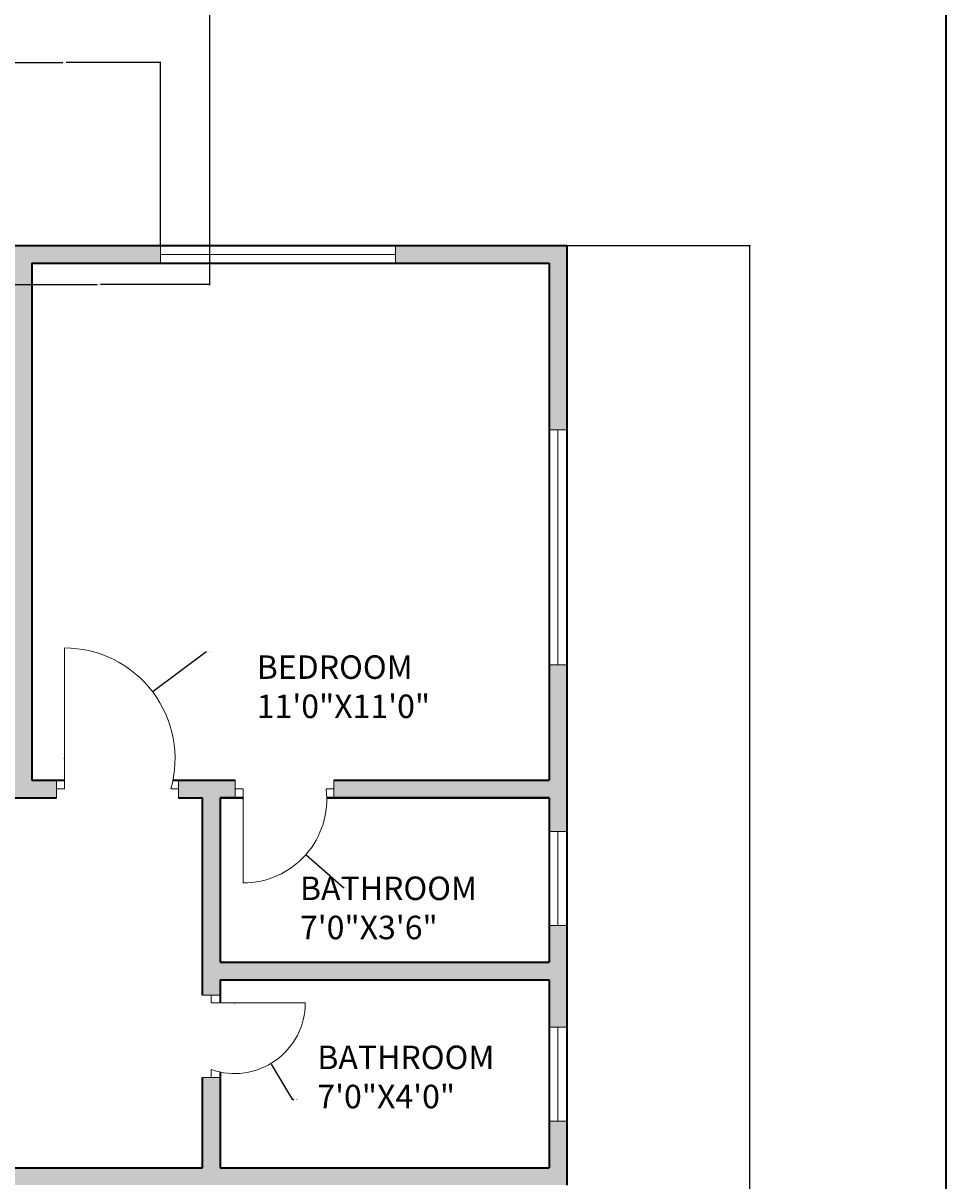
# Model space of a CAD drawing. Units: inches. Extents: x 2314 to 3223, y 1382 to 2735.
# Tile 13 of 14: x 2987 to 3223, y 2143 to 2439. Entities that reach past the tile are written whole.
import ezdxf

# ---------------------------------------------------------------- set-up
doc = ezdxf.new("R2010")
doc.units = ezdxf.units.IN
for name, color, linetype, lineweight in [('A-ANNO-DIMS', 2, 'Continuous', 18), ('A-ANNO-TTLB', 7, 'Continuous', 35), ('A-AREA-IDEN', 7, 'Continuous', 18), ('A-DOOR', 3, 'Continuous', 18), ('A-GLAZ', 4, 'Continuous', 18), ('A-WALL', 7, 'Continuous', 35)]:
    doc.layers.add(name, color=color, linetype=linetype, lineweight=lineweight)
doc.layers.add('A-WALL-PATT', color=251, linetype='Continuous', lineweight=13, true_color=0x636466)
doc.styles.get("Standard").update_dxf_attribs({"font": 'arial.ttf'})
doc.dimstyles.get("Standard").update_dxf_attribs({"dimtxt": 0.18, "dimasz": 0.18, "dimexe": 0.18, "dimexo": 0.0625, "dimgap": 0.09, "dimtad": 0, "dimtih": 1, "dimtoh": 1, "dimdec": 4, "dimzin": 0, "dimdsep": 46, "dimtxsty": 'Standard', "dimcen": 0.09, "dimadec": 0, "dimazin": 0, "dimtfac": 1, "dimtdec": 4, "dimtofl": 0, "dimtmove": 0, "dimatfit": 3, "dimfxl": 1, "dimtolj": 1, "dimtzin": 0, "dimarcsym": 0})

# ---------------------------------------------------------------- blocks, each defined once
blk = doc.blocks.new('WIN-PLAN-24')
for p, q in [((0, 24), (4.5, 24)), ((4.5, 24), (2.25, 24)), ((2.25, 24), (2.25, 0)), ((2.25, 0), (0, 0)), ((0, 0), (4.5, 0))]:
    blk.add_line(p, q)
blk = doc.blocks.new('WIN-PLAN-60')
for p, q in [((0, 4.5), (0, 0)), ((60, 2.25), (60, 4.5)), ((60, 4.5), (60, 0)), ((0, 0), (0, 2.25)), ((0, 2.25), (60, 2.25))]:
    blk.add_line(p, q)
blk = doc.blocks.new('*D30')
at = {"layer": 'A-ANNO-DIMS', "color": 0, "lineweight": -2, "transparency": 16777216}
for p, q in [((3125.96, 2381.78), (3172.77, 2381.78)), ((3172.59, 2381.6), (3172.59, 1973.38)), ((3172.59, 1564.8), (3172.59, 1973.02)), ((2822.96, 1564.62), (3172.77, 1564.62))]:
    blk.add_line(p, q, dxfattribs=at)
at = {"layer": 'A-ANNO-DIMS', "color": 0, "transparency": 16777216}
for points in [[(3172.56, 2381.6), (3172.62, 2381.6), (3172.59, 2381.78)], [(3172.56, 1564.8), (3172.62, 1564.8), (3172.59, 1564.62)]]:
    blk.add_solid(points, dxfattribs=at)
at = {"layer": 'Defpoints', "color": 0, "transparency": 16777216}
for p in [(3125.89, 2381.78), (2822.89, 1564.62), (3172.59, 1564.62)]:
    blk.add_point(p, dxfattribs=at)
at = {"layer": 'A-ANNO-DIMS', "color": 0, "transparency": 16777216, "insert": (3172.59, 1973.2), "char_height": 0.18, "attachment_point": 5}
blk.add_mtext('\\A1;817.2', dxfattribs=at)
blk = doc.blocks.new('*D45')
at = {"layer": 'A-ANNO-DIMS', "color": 0, "lineweight": -2, "transparency": 16777216}
for p, q in [((2973.21, 2381.85), (2973.21, 2428.66)), ((2973.39, 2428.48), (2997.29, 2428.48)), ((3021.98, 2428.48), (2998.08, 2428.48)), ((3022.16, 2381.85), (3022.16, 2428.66))]:
    blk.add_line(p, q, dxfattribs=at)
at = {"layer": 'A-ANNO-DIMS', "color": 0, "transparency": 16777216}
for points in [[(2973.39, 2428.51), (2973.39, 2428.45), (2973.21, 2428.48)], [(3021.98, 2428.51), (3021.98, 2428.45), (3022.16, 2428.48)]]:
    blk.add_solid(points, dxfattribs=at)
at = {"layer": 'Defpoints', "color": 0, "transparency": 16777216}
for p in [(3022.16, 2428.48), (2973.21, 2381.78), (3022.16, 2381.78)]:
    blk.add_point(p, dxfattribs=at)
at = {"layer": 'A-ANNO-DIMS', "color": 0, "transparency": 16777216, "insert": (2997.69, 2428.48), "char_height": 0.18, "attachment_point": 5}
blk.add_mtext('\\A1;48.95', dxfattribs=at)
blk = doc.blocks.new('*D59')
at = {"layer": 'A-ANNO-DIMS', "color": 0, "lineweight": -2, "transparency": 16777216}
for p, q in [((2978.22, 2502.62), (2978.22, 2371.63)), ((3034.7, 2502.62), (3034.7, 2371.63)), ((2978.4, 2371.81), (3006.07, 2371.81)), ((3034.52, 2371.81), (3006.85, 2371.81))]:
    blk.add_line(p, q, dxfattribs=at)
at = {"layer": 'A-ANNO-DIMS', "color": 0, "transparency": 16777216}
for points in [[(2978.4, 2371.84), (2978.4, 2371.78), (2978.22, 2371.81)], [(3034.52, 2371.84), (3034.52, 2371.78), (3034.7, 2371.81)]]:
    blk.add_solid(points, dxfattribs=at)
at = {"layer": 'Defpoints', "color": 0, "transparency": 16777216}
for p in [(2978.22, 2502.68), (3034.7, 2502.68), (3034.7, 2371.81)]:
    blk.add_point(p, dxfattribs=at)
at = {"layer": 'A-ANNO-DIMS', "color": 0, "transparency": 16777216, "insert": (3006.46, 2371.81), "char_height": 0.18, "attachment_point": 5}
blk.add_mtext('\\A1;56.47', dxfattribs=at)
blk = doc.blocks.new('*D74')
at = {"layer": 'A-ANNO-DIMS', "color": 0, "lineweight": -2, "transparency": 16777216}
for p, q in [((3033.74, 2278), (3020.36, 2267.91)), ((3033.92, 2278), (3033.74, 2278)), ((2997.58, 2250.79), (2997.76, 2250.79)), ((2997.67, 2250.7), (2997.67, 2250.88))]:
    blk.add_line(p, q, dxfattribs=at)
at = {"layer": 'A-ANNO-DIMS', "color": 0, "transparency": 16777216}
blk.add_solid([(3020.34, 2267.93), (3020.38, 2267.88), (3020.21, 2267.8)], dxfattribs=at)
at = {"layer": 'Defpoints', "color": 0, "transparency": 16777216}
for p in [(3020.21, 2267.8), (2997.67, 2250.79)]:
    blk.add_point(p, dxfattribs=at)
at = {"layer": 'A-ANNO-DIMS', "color": 0, "transparency": 16777216, "insert": (3034.4, 2278), "char_height": 0.18, "attachment_point": 5}
blk.add_mtext('\\A1;R28.24', dxfattribs=at)
blk = doc.blocks.new('*D86')
at = {"layer": 'A-ANNO-DIMS', "color": 0, "lineweight": -2, "transparency": 16777216}
for p, q in [((3043.27, 2240.32), (3043.27, 2240.5)), ((3043.18, 2240.41), (3043.36, 2240.41)), ((3068.89, 2217.76), (3059.42, 2226.13)), ((3069.07, 2217.76), (3068.89, 2217.76))]:
    blk.add_line(p, q, dxfattribs=at)
at = {"layer": 'A-ANNO-DIMS', "color": 0, "transparency": 16777216}
blk.add_solid([(3059.44, 2226.16), (3059.4, 2226.11), (3059.29, 2226.25)], dxfattribs=at)
at = {"layer": 'Defpoints', "color": 0, "transparency": 16777216}
for p in [(3043.27, 2240.41), (3059.29, 2226.25)]:
    blk.add_point(p, dxfattribs=at)
at = {"layer": 'A-ANNO-DIMS', "color": 0, "transparency": 16777216, "insert": (3069.62, 2217.76), "char_height": 0.18, "attachment_point": 5}
blk.add_mtext('\\A1;R21.375', dxfattribs=at)
blk = doc.blocks.new('*D91')
at = {"layer": 'A-ANNO-DIMS', "color": 0, "lineweight": -2, "transparency": 16777216}
for p, q in [((3041.01, 2188.4), (3041.19, 2188.4)), ((3041.1, 2188.31), (3041.1, 2188.49)), ((3056.02, 2163.69), (3050.52, 2172.8)), ((3056.2, 2163.69), (3056.02, 2163.69))]:
    blk.add_line(p, q, dxfattribs=at)
at = {"layer": 'A-ANNO-DIMS', "color": 0, "transparency": 16777216}
blk.add_solid([(3050.54, 2172.82), (3050.49, 2172.79), (3050.42, 2172.96)], dxfattribs=at)
at = {"layer": 'Defpoints', "color": 0, "transparency": 16777216}
for p in [(3041.1, 2188.4), (3050.42, 2172.96)]:
    blk.add_point(p, dxfattribs=at)
at = {"layer": 'A-ANNO-DIMS', "color": 0, "transparency": 16777216, "insert": (3056.75, 2163.69), "char_height": 0.18, "attachment_point": 5}
blk.add_mtext('\\A1;R18.042', dxfattribs=at)

msp = doc.modelspace()

# ---------------------------------------------------------------- hatches: boundary and pattern name
at = {"layer": 'A-WALL-PATT'}
h = msp.add_hatch(color=256, dxfattribs=at)
h.dxf.hatch_style = 1
h.paths.add_polyline_path([(2443.3302, 2379.5332), (2443.3302, 2381.7832), (2410.3927, 2381.7832), (2410.3927, 2336.7008), (2414.8927, 2336.7008), (2414.8927, 2377.2832), (2443.3302, 2377.2832)])
h.paths.add_polyline_path([(2561.3645, 2379.5332), (2561.3645, 2381.7832), (2503.3302, 2381.7832), (2503.3302, 2377.2832), (2546.8927, 2377.2832), (2546.8927, 2245.2832), (2541.8787, 2245.2832), (2541.8787, 2240.7832), (2551.3927, 2240.7832), (2551.3927, 2377.2832), (2561.3645, 2377.2832)])
h.paths.add_polyline_path([(2656.0607, 2381.7832), (2597.3645, 2381.7832), (2597.3645, 2377.2832), (2617.3927, 2377.2832), (2617.3927, 2257.2832), (2584.2532, 2257.2832), (2584.2532, 2252.7832), (2625.8528, 2252.7832), (2625.8528, 2255.0332), (2625.8528, 2257.2832), (2621.8927, 2257.2832), (2621.8927, 2377.2832), (2656.0607, 2377.2832), (2656.0607, 2379.5332)])
h.paths.add_polyline_path([(2807.3418, 2381.7832), (2716.0607, 2381.7832), (2716.0607, 2377.2832), (2765.8927, 2377.2832), (2765.8927, 2257.2832), (2661.6935, 2257.2832), (2661.6935, 2252.7832), (2765.8927, 2252.7832), (2765.8927, 2146.2832), (2760.9259, 2146.2832), (2760.9259, 2141.8832), (2775.7119, 2141.8832), (2775.7119, 2146.2832), (2770.3927, 2146.2832), (2770.3927, 2252.7832), (2877.684, 2252.7832), (2877.684, 2255.0332), (2877.684, 2257.2832), (2770.3927, 2257.2832), (2770.3927, 2377.2832), (2807.3418, 2377.2832), (2807.3418, 2379.5332)])
h.paths.add_polyline_path([(2937.2118, 2381.7832), (2867.3418, 2381.7832), (2867.3418, 2377.2832), (2914.3927, 2377.2832), (2914.3927, 2257.2832), (2908.4124, 2257.2832), (2908.4124, 2252.7832), (2960.6432, 2252.7832), (2960.6432, 2255.0332), (2960.6432, 2257.2832), (2918.8927, 2257.2832), (2918.8927, 2377.2832), (2937.2118, 2377.2832)])
h.paths.add_polyline_path([(3022.1601, 2381.7832), (2973.2118, 2381.7832), (2973.2118, 2379.5332), (2973.2118, 2377.2832), (2984.8927, 2377.2832), (2984.8927, 2257.2832), (2980.0601, 2257.2832), (2980.0601, 2252.7832), (2984.8927, 2252.7832), (2984.8927, 2240.7832), (2995.668, 2240.7832), (2995.668, 2243.0332), (2995.668, 2245.2832), (2989.3927, 2245.2832), (2989.3927, 2377.2832), (3022.1601, 2377.2832), (3022.1601, 2379.5332)])
h.paths.add_polyline_path([(3125.8927, 2381.7832), (3082.1601, 2381.7832), (3082.1601, 2377.2832), (3121.3927, 2377.2832), (3121.3927, 2334.7388), (3125.8927, 2334.7388)])
h.paths.add_polyline_path([(3125.8927, 2274.7388), (3121.3927, 2274.7388), (3121.3927, 2245.2832), (3066.4832, 2245.2832), (3066.4832, 2240.7832), (3121.3927, 2240.7832), (3121.3927, 2232.1868), (3125.8927, 2232.1868)])
h.paths.add_polyline_path([(3125.8927, 2208.1868), (3121.3927, 2208.1868), (3121.3927, 2198.7832), (3037.3927, 2198.7832), (3037.3927, 2240.7832), (3041.2694, 2240.7832), (3041.2694, 2243.0332), (3041.2694, 2245.2832), (3026.8205, 2245.2832), (3026.8205, 2240.7832), (3032.8927, 2240.7832), (3032.8927, 2190.4022), (3037.3927, 2190.4022), (3037.3927, 2194.2832), (3121.3927, 2194.2832), (3121.3927, 2182.1835), (3125.8927, 2182.1835)])
h.paths.add_polyline_path([(3125.8927, 2158.1835), (3121.3927, 2158.1835), (3121.3927, 2146.2832), (3037.3927, 2146.2832), (3037.3927, 2169.3726), (3035.1427, 2169.3726), (3032.8927, 2169.3726), (3032.8927, 2146.2832), (2812.7301, 2146.2832), (2812.7301, 2144.0832), (2812.7301, 2141.8832), (2818.3927, 2141.8832), (2818.3927, 1970.1316), (2822.8927, 1970.1316), (2822.8927, 1978.8832), (2903.9846, 1978.8832), (2903.9846, 1981.1332), (2903.9846, 1983.3832), (2822.8927, 1983.3832), (2822.8927, 2115.3832), (2851.7162, 2115.3832), (2851.7162, 2117.6332), (2851.7162, 2119.8832), (2822.8927, 2119.8832), (2822.8927, 2141.8832), (3125.8927, 2141.8832)])
h.paths.add_polyline_path([(3125.8927, 2119.8832), (3081.193, 2119.8832), (3081.193, 2115.3832), (3121.3927, 2115.3832), (3121.3927, 2071.8188), (3125.8927, 2071.8188)], flags=17)
h.paths.add_polyline_path([(2989.3927, 2115.3832), (3021.193, 2115.3832), (3021.193, 2117.6332), (3021.193, 2119.8832), (2979.123, 2119.8832), (2979.123, 2115.3832), (2984.8927, 2115.3832), (2984.8927, 2019.3832), (2981.9225, 2019.3832), (2981.9225, 2014.8832), (2984.8927, 2014.8832), (2984.8927, 1983.3832), (2984.8927, 1978.8832), (2989.3927, 1978.8832), (2989.3927, 1983.3832)], flags=17)
h.paths.add_polyline_path([(2947.3927, 2115.3832), (2955.123, 2115.3832), (2955.123, 2117.6332), (2955.123, 2119.8832), (2911.7162, 2119.8832), (2911.7162, 2115.3832), (2942.8927, 2115.3832), (2942.8927, 1983.3832), (2936.7017, 1983.3832), (2936.7017, 1978.8832), (2947.3927, 1978.8832), (2947.3927, 1983.3832), (2947.3927, 2014.8832), (2960.7167, 2014.8832), (2960.7167, 2017.1332), (2960.7167, 2019.3832), (2947.3927, 2019.3832)], flags=17)
h.paths.add_polyline_path([(3037.3927, 1978.8832), (3041.8276, 1978.8832), (3041.8276, 1981.1332), (3041.8276, 1983.3832), (3025.477, 1983.3832), (3025.477, 1978.8832), (3032.8927, 1978.8832), (3032.8927, 1927.1259), (3035.1427, 1927.1259), (3037.3927, 1927.1259)])
h.paths.add_polyline_path([(3125.8927, 2011.8188), (3123.6427, 2011.8188), (3121.3927, 2011.8188), (3121.3927, 1983.3832), (3065, 1983.3832), (3065, 1978.8832), (3121.3927, 1978.8832), (3121.3927, 1970.5932), (3125.8927, 1970.5932)], flags=17)
h.paths.add_polyline_path([(2994.2341, 1983.3832), (2989.3927, 1983.3832), (2989.3927, 1978.8832), (2994.2341, 1978.8832), (2994.2341, 1981.1332)], flags=16)
h.paths.add_polyline_path([(3125.8927, 1946.5932), (3121.3927, 1946.5932), (3121.3927, 1936.8832), (3037.3927, 1936.8832), (3037.3927, 1932.3832), (3121.3927, 1932.3832), (3121.3927, 1919.825), (3125.8927, 1919.825)])
h.paths.add_polyline_path([(3125.8927, 1883.825), (3121.3927, 1883.825), (3121.3927, 1866.3832), (3037.3927, 1866.3832), (3037.3927, 1899.0954), (3035.1427, 1899.0954), (3032.8927, 1899.0954), (3032.8927, 1866.3832), (2822.8927, 1866.3832), (2822.8927, 1938.7212), (2820.6427, 1938.7212), (2818.3927, 1938.7212), (2818.3927, 1786.9239), (2822.8927, 1786.9239), (2822.8927, 1861.8832), (3032.8927, 1861.8832), (3032.8927, 1825.1023), (3037.3927, 1825.1023), (3037.3927, 1861.8832), (3121.3927, 1861.8832), (3121.3927, 1844.6765), (3125.8927, 1844.6765)])
h.paths.add_polyline_path([(3125.8927, 1808.6765), (3121.3927, 1808.6765), (3121.3927, 1795.8832), (3037.3927, 1795.8832), (3037.3927, 1799.4755), (3032.8927, 1799.4755), (3032.8927, 1749.3832), (3026.5034, 1749.3832), (3026.5034, 1744.8832), (3032.8927, 1744.8832), (3034.9255, 1744.8832), (3043.1326, 1744.8832), (3043.1326, 1747.1332), (3043.1326, 1749.3832), (3037.3927, 1749.3832), (3037.3927, 1791.3832), (3121.3927, 1791.3832), (3121.3927, 1783.3103), (3125.8927, 1783.3103)])
h.paths.add_polyline_path([(3125.8927, 1759.3103), (3121.3927, 1759.3103), (3121.3927, 1749.3832), (3065.1845, 1749.3832), (3065.1845, 1744.8832), (3121.3927, 1744.8832), (3121.3927, 1709.3573), (3125.8927, 1709.3573)])
h.paths.add_polyline_path([(3125.8927, 1649.3573), (3121.3927, 1649.3573), (3121.3927, 1612.8832), (3095.116, 1612.8832), (3095.116, 1608.3832), (3125.8927, 1608.3832)])
h.paths.add_polyline_path([(3035.116, 1612.8832), (2993.8927, 1612.8832), (2993.8927, 1744.8832), (2998.7409, 1744.8832), (2998.7409, 1749.3832), (2989.3927, 1749.3832), (2989.3927, 1744.8832), (2989.3927, 1701.3832), (2972.8226, 1701.3832), (2972.8226, 1696.8832), (2989.3927, 1696.8832), (2989.3927, 1612.8832), (2978.2225, 1612.8832), (2978.2225, 1608.3832), (3035.116, 1608.3832), (3035.116, 1610.6332)])
h.paths.add_polyline_path([(2947.3927, 1696.8832), (2950.7566, 1696.8832), (2950.7566, 1699.1332), (2950.7566, 1701.3832), (2947.3927, 1701.3832), (2947.3927, 1744.8832), (2947.3927, 1749.3832), (2937.649, 1749.3832), (2937.649, 1744.8832), (2942.8927, 1744.8832), (2942.8927, 1612.8832), (2907.783, 1612.8832), (2907.783, 1608.3832), (2954.2225, 1608.3832), (2954.2225, 1610.6332), (2954.2225, 1612.8832), (2947.3927, 1612.8832)])
h.paths.add_polyline_path([(2822.8927, 1744.8832), (2905.3491, 1744.8832), (2905.3491, 1747.1332), (2905.3491, 1749.3832), (2822.8927, 1749.3832), (2822.8927, 1756.9185), (2818.3927, 1756.9185), (2818.3927, 1612.8832), (2818.3927, 1569.1205), (2722.3927, 1569.1205), (2722.3927, 1612.8832), (2722.3927, 1756.9185), (2717.8927, 1756.9185), (2717.8927, 1750.0143), (2633.6297, 1750.0143), (2633.6437, 1745.2665), (2717.8927, 1745.5143), (2717.8927, 1612.8832), (2689.8467, 1612.8832), (2689.8467, 1608.3832), (2717.8927, 1608.3832), (2717.8927, 1564.6205), (2722.3927, 1564.6205), (2822.8927, 1564.6205), (2822.8927, 1569.1205), (2822.8927, 1608.3832), (2847.783, 1608.3832), (2847.783, 1610.6332), (2847.783, 1612.8832), (2822.8927, 1612.8832)])
h.paths.add_polyline_path([(2629.8467, 1612.8832), (2597.8927, 1612.8832), (2597.8927, 1744.8832), (2597.8927, 1745.1613), (2601.5887, 1745.1721), (2601.5816, 1747.5932), (2601.5745, 1750.0143), (2593.3927, 1750.0143), (2593.3927, 1744.8832), (2593.3927, 1713.3832), (2589.7588, 1713.3832), (2589.7588, 1708.8832), (2593.3927, 1708.8832), (2593.3927, 1612.8832), (2582.3793, 1612.8832), (2582.3793, 1608.3832), (2629.8467, 1608.3832), (2629.8467, 1610.6332)])
h.paths.add_polyline_path([(2551.3927, 1708.8832), (2567.6776, 1708.8832), (2567.6776, 1711.1332), (2567.6776, 1713.3832), (2551.3927, 1713.3832), (2551.3927, 1744.8832), (2551.3927, 1750.0143), (2543.5657, 1750.0143), (2543.5657, 1747.5079), (2543.5657, 1745.0014), (2546.8927, 1745.0112), (2546.8927, 1744.8832), (2546.8927, 1612.8832), (2502.9339, 1612.8832), (2502.9339, 1608.3832), (2558.3793, 1608.3832), (2558.3793, 1610.6332), (2558.3793, 1612.8832), (2551.3927, 1612.8832)])
h.paths.add_polyline_path([(2414.8927, 1656.2547), (2410.3927, 1656.2547), (2410.3927, 1608.3832), (2442.9339, 1608.3832), (2442.9339, 1610.6332), (2442.9339, 1612.8832), (2414.8927, 1612.8832)])
h.paths.add_polyline_path([(2414.8927, 1744.8832), (2468.8906, 1744.8832), (2468.8906, 1747.1332), (2468.8906, 1749.3832), (2414.8927, 1749.3832), (2414.8927, 1757.7622), (2410.3927, 1757.7622), (2410.3927, 1716.2547), (2414.8927, 1716.2547)])
h.paths.add_polyline_path([(2414.8927, 1791.3832), (2498.8927, 1791.3832), (2498.8927, 1749.3832), (2492.9799, 1749.3832), (2492.9799, 1744.8832), (2498.8927, 1744.8832), (2503.3927, 1744.8832), (2508.0135, 1744.8968), (2508.0059, 1747.4556), (2507.9984, 1750.0143), (2503.3927, 1750.0143), (2503.3927, 1802.6362), (2501.1427, 1802.6362), (2498.8927, 1802.6362), (2498.8927, 1795.8832), (2414.8927, 1795.8832), (2414.8927, 1808.0943), (2410.3927, 1808.0943), (2410.3927, 1781.7622), (2414.8927, 1781.7622)])
h.paths.add_polyline_path([(2722.3927, 1937.589), (2720.1427, 1937.589), (2717.8927, 1937.589), (2717.8927, 1866.3832), (2503.3927, 1866.3832), (2503.3927, 1896.3484), (2498.8927, 1896.3484), (2498.8927, 1866.3832), (2414.8927, 1866.3832), (2414.8927, 1882.1496), (2410.3927, 1882.1496), (2410.3927, 1844.0943), (2414.8927, 1844.0943), (2414.8927, 1861.8832), (2498.8927, 1861.8832), (2498.8927, 1831.4783), (2501.1427, 1831.4783), (2503.3927, 1831.4783), (2503.3927, 1861.8832), (2717.8927, 1861.8832), (2717.8927, 1786.9239), (2722.3927, 1786.9239)])
h.paths.add_polyline_path([(2414.8927, 1932.3832), (2498.8927, 1932.3832), (2498.8927, 1924.7883), (2503.3927, 1924.7883), (2503.3927, 1978.8832), (2505.8599, 1978.8832), (2505.8599, 1981.1332), (2505.8599, 1983.3832), (2493.3697, 1983.3832), (2493.3697, 1978.8832), (2498.8927, 1978.8832), (2498.8927, 1936.8832), (2414.8927, 1936.8832), (2414.8927, 1943.2834), (2410.3927, 1943.2834), (2410.3927, 1918.1496), (2414.8927, 1918.1496)])
h.paths.add_polyline_path([(2414.8927, 2020.3133), (2412.6427, 2020.3133), (2410.3927, 2020.3133), (2410.3927, 1967.2834), (2414.8927, 1967.2834), (2414.8927, 1978.8832), (2468.8513, 1978.8832), (2468.8513, 1981.1332), (2468.8513, 1983.3832), (2414.8927, 1983.3832)])
h.paths.add_polyline_path([(2414.8927, 2115.3832), (2453.004, 2115.3832), (2453.004, 2117.6332), (2453.004, 2119.8832), (2410.3927, 2119.8832), (2410.3927, 2080.3133), (2414.8927, 2080.3133)], flags=17)
h.paths.add_polyline_path([(2559.0969, 2117.6332), (2559.0969, 2119.8832), (2513.004, 2119.8832), (2513.004, 2115.3832), (2546.8927, 2115.3832), (2546.8927, 1983.3832), (2542.7531, 1983.3832), (2542.7531, 1978.8832), (2551.3927, 1978.8832), (2551.3927, 2014.8832), (2570.3098, 2014.8832), (2570.3098, 2017.1332), (2570.3098, 2019.3832), (2551.3927, 2019.3832), (2551.3927, 2115.3832), (2559.0969, 2115.3832)], flags=17)
h.paths.add_polyline_path([(2628.5073, 2117.6332), (2628.5073, 2119.8832), (2583.0969, 2119.8832), (2583.0969, 2115.3832), (2593.3927, 2115.3832), (2593.3927, 2019.3832), (2590.2108, 2019.3832), (2590.2108, 2014.8832), (2593.3927, 2014.8832), (2593.3927, 1978.8832), (2601.5907, 1978.8832), (2601.5907, 1981.1332), (2601.5907, 1983.3832), (2597.8927, 1983.3832), (2597.8927, 2115.3832), (2628.5073, 2115.3832)], flags=17)
h.paths.add_polyline_path([(2722.3927, 2141.8832), (2726.9871, 2141.8832), (2726.9871, 2144.2705), (2726.9871, 2146.2832), (2503.3927, 2146.2832), (2503.3927, 2168.2161), (2501.1427, 2168.2161), (2498.8927, 2168.2161), (2498.8927, 2146.2832), (2414.8927, 2146.2832), (2414.8927, 2156.5041), (2410.3927, 2156.5041), (2410.3927, 2141.8832), (2717.8927, 2141.8832), (2717.8927, 2119.8832), (2688.5073, 2119.8832), (2688.5073, 2115.3832), (2717.8927, 2115.3832), (2717.8927, 1983.3832), (2633.2454, 1983.3832), (2633.2454, 1978.8832), (2717.8927, 1978.8832), (2717.8927, 1970.1316), (2720.1427, 1970.1316), (2722.3927, 1970.1316)])
h.paths.add_polyline_path([(2557.3704, 1462.9278), (2940.0934, 1462.9278), (2940.0934, 1512.3848), (2557.3704, 1512.3848)], flags=9)
h.paths.add_polyline_path([(2846.2527, 1703.1384), (2892.8612, 1703.1384), (2892.8612, 1725.5272), (2846.2527, 1725.5272)], flags=25)
h.paths.add_polyline_path([(2885.6102, 1812.1147), (2946.1505, 1812.1147), (2946.1505, 1834.5035), (2885.6102, 1834.5035)], flags=25)
h.paths.add_polyline_path([(2885.6102, 1884.183), (2946.1505, 1884.183), (2946.1505, 1906.5718), (2885.6102, 1906.5718)], flags=25)
h.paths.add_polyline_path([(3066.365, 1705.5431), (3112.9735, 1705.5431), (3112.9735, 1727.9319), (3066.365, 1727.9319)], flags=9)
h.paths.add_polyline_path([(3061.8255, 1887.7513), (3101.6154, 1887.7513), (3101.6154, 1910.1401), (3061.8255, 1910.1401)], flags=25)
h.paths.add_polyline_path([(3063.3679, 1816.2121), (3103.1578, 1816.2121), (3103.1578, 1838.6009), (3063.3679, 1838.6009)], flags=25)
h.paths.add_polyline_path([(3053.3743, 1768.416), (3107.1329, 1768.416), (3107.1329, 1790.8048), (3053.3743, 1790.8048)], flags=25)
h.paths.add_polyline_path([(3061.6068, 1943.822), (3115.3653, 1943.822), (3115.3653, 1966.2109), (3061.6068, 1966.2109)], flags=9)
h.paths.add_polyline_path([(2745.0978, 1763.6604), (2797.9354, 1763.6604), (2797.9354, 1776.0247), (2745.0978, 1776.0247)], flags=9)
h.paths.add_polyline_path([(2574.2135, 1819.2586), (2634.7538, 1819.2586), (2634.7538, 1841.6474), (2574.2135, 1841.6474)], flags=25)
h.paths.add_polyline_path([(2574.2135, 1891.3269), (2634.7538, 1891.3269), (2634.7538, 1913.7157), (2574.2135, 1913.7157)], flags=25)
h.paths.add_polyline_path([(2638.4466, 1702.43), (2685.0551, 1702.43), (2685.0551, 1724.8188), (2638.4466, 1724.8188)], flags=25)
h.paths.add_polyline_path([(2435.9715, 1697.1215), (2482.5799, 1697.1215), (2482.5799, 1719.5103), (2435.9715, 1719.5103)], flags=9)
h.paths.add_polyline_path([(2431.2046, 1893.7833), (2470.9945, 1893.7833), (2470.9945, 1916.1721), (2431.2046, 1916.1721)], flags=25)
h.paths.add_polyline_path([(2439.8144, 1817.2116), (2479.6043, 1817.2116), (2479.6043, 1839.6004), (2439.8144, 1839.6004)], flags=25)
h.paths.add_polyline_path([(2441.2607, 1753.0942), (2495.0192, 1753.0942), (2495.0192, 1775.483), (2441.2607, 1775.483)], flags=25)
h.paths.add_polyline_path([(2421.216, 1945.3109), (2474.9746, 1945.3109), (2474.9746, 1967.6997), (2421.216, 1967.6997)], flags=25)
h.paths.add_polyline_path([(2585.4464, 1627.5703), (2585.4464, 1679), (2563.0576, 1679), (2563.0576, 1627.5703)], flags=9)
h.paths.add_polyline_path([(2978.3497, 1618.7039), (2978.3497, 1670.1337), (2955.9609, 1670.1337), (2955.9609, 1618.7039)], flags=9)
h.paths.add_polyline_path([(2975.9502, 2041.7828), (2975.9502, 2093.2125), (2953.5614, 2093.2125), (2953.5614, 2041.7828)], flags=25)
h.paths.add_polyline_path([(2835.6537, 1989.2068), (2882.2621, 1989.2068), (2882.2621, 2011.5956), (2835.6537, 2011.5956)], flags=25)
h.paths.add_polyline_path([(2649.3769, 1997.5659), (2695.9853, 1997.5659), (2695.9853, 2019.9547), (2649.3769, 2019.9547)], flags=25)
h.paths.add_polyline_path([(2579.9087, 2040.3429), (2579.9087, 2091.7726), (2557.5198, 2091.7726), (2557.5198, 2040.3429)], flags=25)
h.paths.add_polyline_path([(2783.2404, 1883.1956), (2783.2404, 2067.1369), (2764.694, 2067.1369), (2764.694, 1883.1956)], flags=9)
h.paths.add_polyline_path([(3055.8435, 1993.5571), (3102.4519, 1993.5571), (3102.4519, 2015.9459), (3055.8435, 2015.9459)], flags=25)
h.paths.add_polyline_path([(2423.6009, 1984.6082), (2470.2094, 1984.6082), (2470.2094, 2006.997), (2423.6009, 2006.997)], flags=25)
h.paths.add_polyline_path([(2973.4115, 2123.1668), (3013.1319, 2123.1668), (3013.1319, 2135.531), (2973.4115, 2135.531)], flags=25)
h.paths.add_polyline_path([(2534.3846, 2124.6231), (2574.105, 2124.6231), (2574.105, 2136.9874), (2534.3846, 2136.9874)], flags=25)
h.paths.add_polyline_path([(2829.1368, 2188.1931), (2889.411, 2188.1931), (2889.411, 2210.5819), (2829.1368, 2210.5819)], flags=9)
h.paths.add_polyline_path([(2633.2547, 2185.0437), (2693.5289, 2185.0437), (2693.5289, 2207.4325), (2633.2547, 2207.4325)], flags=9)
h.paths.add_polyline_path([(2445.1812, 2167.0395), (2496.611, 2167.0395), (2496.611, 2189.4284), (2445.1812, 2189.4284)], flags=9)
h.paths.add_polyline_path([(2429.1678, 2194.5482), (2480.5975, 2194.5482), (2480.5975, 2216.937), (2429.1678, 2216.937)], flags=9)
h.paths.add_polyline_path([(3060.1138, 2158.1056), (3111.5436, 2158.1056), (3111.5436, 2180.4944), (3060.1138, 2180.4944)], flags=9)
h.paths.add_polyline_path([(3055.6824, 2201.2631), (3107.1122, 2201.2631), (3107.1122, 2223.652), (3055.6824, 2223.652)], flags=25)
h.paths.add_polyline_path([(3044.3482, 2257.7345), (3090.9567, 2257.7345), (3090.9567, 2280.1233), (3044.3482, 2280.1233)], flags=9)
h.paths.add_polyline_path([(2942.5437, 2306.9625), (2982.3336, 2306.9625), (2982.3336, 2329.3513), (2942.5437, 2329.3513)], flags=9)
h.paths.add_polyline_path([(2799.5865, 2259.1663), (2846.195, 2259.1663), (2846.195, 2281.5551), (2799.5865, 2281.5551)], flags=25)
h.paths.add_polyline_path([(2670.4998, 2261.1493), (2717.1082, 2261.1493), (2717.1082, 2283.5381), (2670.4998, 2283.5381)], flags=25)
h.paths.add_polyline_path([(2553.0333, 2302.7735), (2592.8232, 2302.7735), (2592.8232, 2325.1624), (2553.0333, 2325.1624)], flags=9)
h.paths.add_polyline_path([(2432.0288, 2268.6489), (2478.6372, 2268.6489), (2478.6372, 2291.0377), (2432.0288, 2291.0377)], flags=9)
h = msp.add_hatch(color=256, dxfattribs=at)
h.dxf.hatch_style = 1
h.paths.add_polyline_path([(2503.3927, 2240.7832), (2507.7952, 2240.7832), (2507.7952, 2245.2832), (2496.4262, 2245.2832), (2496.4262, 2243.0332), (2496.4262, 2240.7832), (2498.8927, 2240.7832), (2498.8927, 2198.7832), (2414.8927, 2198.7832), (2414.8927, 2206.5718), (2410.3927, 2206.5718), (2410.3927, 2180.5041), (2412.6427, 2180.5041), (2414.8927, 2180.5041), (2414.8927, 2194.2832), (2498.8927, 2194.2832), (2498.8927, 2191.0069), (2503.3927, 2191.0069)])
h.paths.add_polyline_path([(2414.8927, 2276.7008), (2410.3927, 2276.7008), (2410.3927, 2230.5718), (2414.8927, 2230.5718), (2414.8927, 2240.7832), (2474.2564, 2240.7832), (2474.2564, 2243.0332), (2474.2564, 2245.2832), (2414.8927, 2245.2832)])
h.paths.add_polyline_path([(2557.3704, 1462.9278), (2940.0934, 1462.9278), (2940.0934, 1512.3848), (2557.3704, 1512.3848)], flags=9)
h.paths.add_polyline_path([(2846.2527, 1703.1384), (2892.8612, 1703.1384), (2892.8612, 1725.5272), (2846.2527, 1725.5272)], flags=9)
h.paths.add_polyline_path([(2885.6102, 1812.1147), (2946.1505, 1812.1147), (2946.1505, 1834.5035), (2885.6102, 1834.5035)], flags=9)
h.paths.add_polyline_path([(2885.6102, 1884.183), (2946.1505, 1884.183), (2946.1505, 1906.5718), (2885.6102, 1906.5718)], flags=9)
h.paths.add_polyline_path([(3066.365, 1705.5431), (3112.9735, 1705.5431), (3112.9735, 1727.9319), (3066.365, 1727.9319)], flags=9)
h.paths.add_polyline_path([(3061.8255, 1887.7513), (3101.6154, 1887.7513), (3101.6154, 1910.1401), (3061.8255, 1910.1401)], flags=9)
h.paths.add_polyline_path([(3063.3679, 1816.2121), (3103.1578, 1816.2121), (3103.1578, 1838.6009), (3063.3679, 1838.6009)], flags=9)
h.paths.add_polyline_path([(3053.3743, 1768.416), (3107.1329, 1768.416), (3107.1329, 1790.8048), (3053.3743, 1790.8048)], flags=9)
h.paths.add_polyline_path([(3061.6068, 1943.822), (3115.3653, 1943.822), (3115.3653, 1966.2109), (3061.6068, 1966.2109)], flags=9)
h.paths.add_polyline_path([(2745.0978, 1763.6604), (2797.9354, 1763.6604), (2797.9354, 1776.0247), (2745.0978, 1776.0247)], flags=9)
h.paths.add_polyline_path([(2574.2135, 1819.2586), (2634.7538, 1819.2586), (2634.7538, 1841.6474), (2574.2135, 1841.6474)], flags=9)
h.paths.add_polyline_path([(2574.2135, 1891.3269), (2634.7538, 1891.3269), (2634.7538, 1913.7157), (2574.2135, 1913.7157)], flags=9)
h.paths.add_polyline_path([(2638.4466, 1702.43), (2685.0551, 1702.43), (2685.0551, 1724.8188), (2638.4466, 1724.8188)], flags=9)
h.paths.add_polyline_path([(2435.9715, 1697.1215), (2482.5799, 1697.1215), (2482.5799, 1719.5103), (2435.9715, 1719.5103)], flags=9)
h.paths.add_polyline_path([(2431.2046, 1893.7833), (2470.9945, 1893.7833), (2470.9945, 1916.1721), (2431.2046, 1916.1721)], flags=9)
h.paths.add_polyline_path([(2439.8144, 1817.2116), (2479.6043, 1817.2116), (2479.6043, 1839.6004), (2439.8144, 1839.6004)], flags=9)
h.paths.add_polyline_path([(2441.2607, 1753.0942), (2495.0192, 1753.0942), (2495.0192, 1775.483), (2441.2607, 1775.483)], flags=9)
h.paths.add_polyline_path([(2421.216, 1945.3109), (2474.9746, 1945.3109), (2474.9746, 1967.6997), (2421.216, 1967.6997)], flags=9)
h.paths.add_polyline_path([(2585.4464, 1627.5703), (2585.4464, 1679), (2563.0576, 1679), (2563.0576, 1627.5703)], flags=9)
h.paths.add_polyline_path([(2978.3497, 1618.7039), (2978.3497, 1670.1337), (2955.9609, 1670.1337), (2955.9609, 1618.7039)], flags=9)
h.paths.add_polyline_path([(2975.9502, 2041.7828), (2975.9502, 2093.2125), (2953.5614, 2093.2125), (2953.5614, 2041.7828)], flags=9)
h.paths.add_polyline_path([(2835.6537, 1989.2068), (2882.2621, 1989.2068), (2882.2621, 2011.5956), (2835.6537, 2011.5956)], flags=9)
h.paths.add_polyline_path([(2649.3769, 1997.5659), (2695.9853, 1997.5659), (2695.9853, 2019.9547), (2649.3769, 2019.9547)], flags=9)
h.paths.add_polyline_path([(2579.9087, 2040.3429), (2579.9087, 2091.7726), (2557.5198, 2091.7726), (2557.5198, 2040.3429)], flags=9)
h.paths.add_polyline_path([(2783.2404, 1883.1956), (2783.2404, 2067.1369), (2764.694, 2067.1369), (2764.694, 1883.1956)], flags=9)
h.paths.add_polyline_path([(3055.8435, 1993.5571), (3102.4519, 1993.5571), (3102.4519, 2015.9459), (3055.8435, 2015.9459)], flags=9)
h.paths.add_polyline_path([(2423.6009, 1984.6082), (2470.2094, 1984.6082), (2470.2094, 2006.997), (2423.6009, 2006.997)], flags=9)
h.paths.add_polyline_path([(2973.4115, 2123.1668), (3013.1319, 2123.1668), (3013.1319, 2135.531), (2973.4115, 2135.531)], flags=9)
h.paths.add_polyline_path([(2534.3846, 2124.6231), (2574.105, 2124.6231), (2574.105, 2136.9874), (2534.3846, 2136.9874)], flags=9)
h.paths.add_polyline_path([(2829.1368, 2188.1931), (2889.411, 2188.1931), (2889.411, 2210.5819), (2829.1368, 2210.5819)], flags=9)
h.paths.add_polyline_path([(2633.2547, 2185.0437), (2693.5289, 2185.0437), (2693.5289, 2207.4325), (2633.2547, 2207.4325)], flags=9)
h.paths.add_polyline_path([(2445.1812, 2167.0395), (2496.611, 2167.0395), (2496.611, 2189.4284), (2445.1812, 2189.4284)], flags=9)
h.paths.add_polyline_path([(2429.1678, 2208.3022), (2480.5975, 2208.3022), (2480.5975, 2230.691), (2429.1678, 2230.691)], flags=25)
h.paths.add_polyline_path([(3060.1138, 2158.1056), (3111.5436, 2158.1056), (3111.5436, 2180.4944), (3060.1138, 2180.4944)], flags=9)
h.paths.add_polyline_path([(3055.6824, 2201.2631), (3107.1122, 2201.2631), (3107.1122, 2223.652), (3055.6824, 2223.652)], flags=9)
h.paths.add_polyline_path([(3044.3482, 2257.7345), (3090.9567, 2257.7345), (3090.9567, 2280.1233), (3044.3482, 2280.1233)], flags=9)
h.paths.add_polyline_path([(2942.5437, 2306.9625), (2982.3336, 2306.9625), (2982.3336, 2329.3513), (2942.5437, 2329.3513)], flags=9)
h.paths.add_polyline_path([(2799.5865, 2259.1663), (2846.195, 2259.1663), (2846.195, 2281.5551), (2799.5865, 2281.5551)], flags=9)
h.paths.add_polyline_path([(2670.4998, 2261.1493), (2717.1082, 2261.1493), (2717.1082, 2283.5381), (2670.4998, 2283.5381)], flags=9)
h.paths.add_polyline_path([(2553.0333, 2302.7735), (2592.8232, 2302.7735), (2592.8232, 2325.1624), (2553.0333, 2325.1624)], flags=9)
h.paths.add_polyline_path([(2432.0288, 2268.6489), (2478.6372, 2268.6489), (2478.6372, 2291.0377), (2432.0288, 2291.0377)], flags=9)

# ---------------------------------------------------------------- linework, layer by layer
at = {"layer": 'A-ANNO-TTLB'}
msp.add_lwpolyline([(2314.008, 2735.417), (3222.6676, 2735.417), (3222.6676, 1382.0876), (2314.008, 1382.0876)], close=True, dxfattribs=at)
at = {"layer": 'A-DOOR'}
for p, q in [((2997.668, 2243.0332), (2997.668, 2279.0332)), ((2995.668, 2245.2832), (2995.668, 2240.7832)), ((3026.8205, 2245.2832), (3026.8205, 2240.7832)), ((3041.2694, 2245.2832), (3041.2694, 2240.7832)), ((3066.4832, 2245.2832), (3066.4832, 2240.7832)), ((2995.668, 2240.7832), (2995.668, 2243.0332)), ((2995.668, 2243.0332), (2997.668, 2243.0332)), ((3026.8205, 2243.0332), (3024.8205, 2243.0332)), ((3026.8205, 2240.7832), (3026.8205, 2243.0332)), ((3041.2694, 2240.7832), (3041.2694, 2243.0332)), ((3041.2694, 2243.0332), (3043.2694, 2243.0332)), ((3043.2694, 2243.0332), (3043.2694, 2219.0332)), ((3066.4832, 2243.0332), (3064.4832, 2243.0332)), ((3066.4832, 2240.7832), (3066.4832, 2243.0332)), ((3032.8927, 2190.4022), (3037.3927, 2190.4022)), ((3037.3927, 2190.4022), (3035.1427, 2190.4022)), ((3035.1427, 2190.4022), (3035.1427, 2188.4022)), ((3035.1427, 2188.4022), (3059.1427, 2188.4022)), ((3035.1427, 2169.3726), (3035.1427, 2171.3726)), ((3032.8927, 2169.3726), (3037.3927, 2169.3726)), ((3037.3927, 2169.3726), (3035.1427, 2169.3726))]:
    msp.add_line(p, q, dxfattribs=at)
for centre, radius, start, end in [((2997.668, 2250.7935), 28.2397, 344.049902, 90), ((3043.2694, 2240.4087), 21.3755, 270, 7.05274), ((3041.1008, 2188.4022), 18.0418, 250.716558, 0)]:
    msp.add_arc(centre, radius, start, end, dxfattribs=at)
at = {"layer": 'A-WALL'}
for p, q in [((2410.3927, 2381.7832), (3125.8927, 2381.7832)), ((3125.8927, 2381.7832), (3125.8927, 2141.8832)), ((2989.3927, 2377.2832), (2989.3927, 2245.2832)), ((2989.3927, 2377.2832), (3121.3927, 2377.2832)), ((3121.3927, 2377.2832), (3121.3927, 2245.2832)), ((2989.3927, 2245.2832), (2997.668, 2245.2832)), ((3025.3649, 2245.2832), (3041.2694, 2245.2832)), ((3066.4832, 2245.2832), (3121.3927, 2245.2832)), ((2984.8927, 2240.7832), (2995.668, 2240.7832)), ((3026.8205, 2240.7832), (3032.8927, 2240.7832)), ((3032.8927, 2190.4022), (3032.8927, 2240.7832)), ((3037.3927, 2240.7832), (3037.3927, 2198.7832)), ((3043.2694, 2240.7832), (3037.3927, 2240.7832)), ((3037.3927, 2240.7832), (3043.2694, 2240.7832)), ((3121.3927, 2240.7832), (3064.6416, 2240.7832)), ((3064.6416, 2240.7832), (3121.3927, 2240.7832)), ((3121.3927, 2240.7832), (3121.3927, 2198.7832)), ((3037.3927, 2198.7832), (3121.3927, 2198.7832)), ((3037.3927, 2194.2832), (3037.3927, 2188.4022)), ((3037.3927, 2194.2832), (3121.3927, 2194.2832)), ((3121.3927, 2194.2832), (3121.3927, 2146.2832)), ((3037.3927, 2170.7455), (3037.3927, 2146.2832)), ((3032.8927, 2146.2832), (3032.8927, 2169.3726)), ((2810.847, 2146.2832), (3032.8927, 2146.2832)), ((3037.3927, 2146.2832), (3121.3927, 2146.2832))]:
    msp.add_line(p, q, dxfattribs=at)

# ---------------------------------------------------------------- block references
at = {"layer": 'A-GLAZ', "rotation": 180}
for name, p in [('WIN-PLAN-60', (3082.1601, 2381.7832)), ('WIN-PLAN-24', (3125.8927, 2232.1868)), ('WIN-PLAN-24', (3125.8927, 2182.1835))]:
    msp.add_blockref(name, p, dxfattribs=at)
at = {"layer": 'A-GLAZ', "extrusion": (0, 0, -1), "zscale": -1, "rotation": 90}
msp.add_blockref('WIN-PLAN-60', (-3121.3927, 2274.7388), dxfattribs=at)

# ---------------------------------------------------------------- texts
at = {"layer": 'A-AREA-IDEN', "char_height": 6, "attachment_point": 1}
for s, width, insert in [('BEDROOM\\P11\'0"X11\'0"', 116.951221, (3046.7609, 2277.1417)), ('BATHROOM\\P7\'0"X3\'6"', 110.597382, (3057.7963, 2220.6704)), ('BATHROOM\\P7\'0"X4\'0"', 110.597382, (3062.2278, 2177.5128))]:
    msp.add_mtext_dynamic_manual_height_columns(s, width=width, gutter_width=12.5, heights=[0], dxfattribs=dict(at, insert=insert))

# ---------------------------------------------------------------- dimensions: what is measured, and where the dimension line sits
at = {"layer": 'A-ANNO-DIMS'}
for base, p1, p2, picture, middle in [((3034.6958, 2371.8121), (2978.2225, 2502.6793), (3034.6958, 2502.6793), '*D59', (3006.4592, 2371.8121)), ((3022.1601, 2428.4832), (2973.2118, 2381.7832), (3022.1601, 2381.7832), '*D45', (2997.686, 2428.4832))]:
    dim = msp.add_linear_dim(base=base, p1=p1, p2=p2, dimstyle='Standard', override={"dimdec": 2, "dimlfac": 1, "dimrnd": 0, "dimzin": 0, "dimdsep": 46, "dimlunit": 2}, dxfattribs=at)
    dim.commit()
    dim.dimension.update_dxf_attribs({"geometry": picture, "text_midpoint": middle})
dim = msp.add_linear_dim(base=(3172.5927, 1564.6205), p1=(3125.8927, 2381.7832), p2=(2822.8927, 1564.6205), angle=90, dimstyle='Standard', override={"dimdec": 1, "dimlfac": 1, "dimrnd": 0, "dimzin": 0, "dimdsep": 46, "dimlunit": 2}, dxfattribs=at)
dim.commit()
dim.dimension.update_dxf_attribs({"geometry": '*D30', "text_midpoint": (3172.5927, 1973.2019)})
for center, mpoint, override, picture, middle in [((2997.668, 2250.7935), (3020.2141, 2267.7981), {"dimdec": 2, "dimlfac": 1, "dimrnd": 0, "dimzin": 0, "dimdsep": 46, "dimlunit": 2}, '*D74', (3034.4012, 2278.0008)), ((3043.2694, 2240.4087), (3059.285, 2226.252), {"dimdec": 3, "dimlfac": 1, "dimrnd": 0, "dimzin": 0, "dimdsep": 46, "dimlunit": 2}, '*D86', (3069.6248, 2217.758)), ((3041.1008, 2188.4022), (3050.4233, 2172.9555), {"dimdec": 3, "dimlfac": 1, "dimrnd": 0, "dimzin": 0, "dimdsep": 46, "dimlunit": 2}, '*D91', (3056.7456, 2163.6875))]:
    dim = msp.add_radius_dim(center=center, mpoint=mpoint, dimstyle='Standard', override=override, dxfattribs=at)
    dim.commit()
    dim.dimension.update_dxf_attribs({"geometry": picture, "text_midpoint": middle, "dimtype": 164})

doc.saveas('drawing.dxf')
